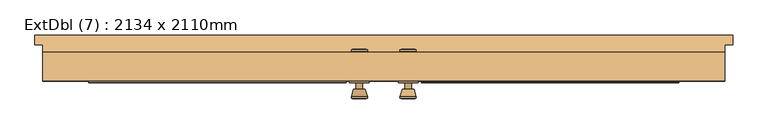
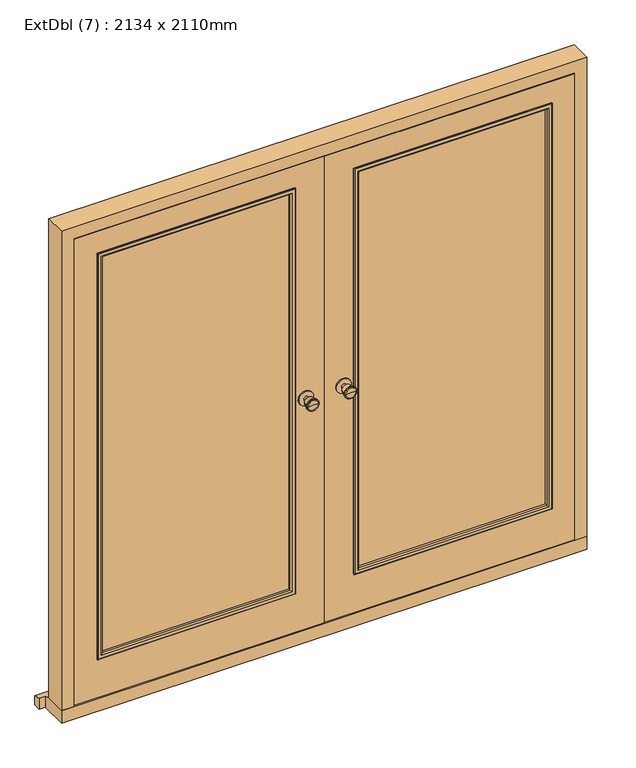
"""IFC4 building model written with IfcOpenShell, lengths in millimetres: door geometry, ExtDbl (7) : 2134 x 2110mm."""

from ifc_helpers import new_model, si_unit, point, frame, frame_2d, origin, place, context, project, spatial, polyline, circle_curve, ellipse_curve, trimmed, segment, composite_curve, outline, extrude, faceted_brep, source, transform, mapped, element, save
from ifc_brep_helpers import plane_surface, cylinder_surface, revolved_surface, advanced_brep


def extdbl_7_2134_x_2110mm_9b31339b(model_context):
    return source(origin(), model_context, "Body", "SolidModel", [
        advanced_brep(
        [(-76.5, -5.7, 1050.0), (-66.5, -5.7, 1050.0), (-86.5, -5.7, 1050.0), (-96.9758676, -54.7, 1050.0), (-56.0241324, -54.7, 1050.0), (-76.5, -54.7, 1050.0), (-101.5, -52.8721319, 1050.0), (-51.5, -52.8721319, 1050.0), (-101.5, -49.4084537, 1050.0), (-51.5, -49.4084537, 1050.0), (-95.136236, -24.7, 1050.0), (-57.863764, -24.7, 1050.0), (-86.5, -24.7, 1050.0), (-66.5, -24.7, 1050.0)],
        [
            (0, 1),
            (1, 2, circle_curve(frame((-76.5, -5.7, 1050.0), z_axis=(0.0, 1.0, 0.0), x_axis=(1.0, 0.0, 0.0)), 10.0)),
            (2, 0),
            (2, 1, circle_curve(frame((-76.5, -5.7, 1050.0), z_axis=(0.0, 1.0, 0.0), x_axis=(1.0, 0.0, 0.0)), 10.0)),
            (3, 4, circle_curve(frame((-76.5, -54.7, 1050.0), z_axis=(0.0, -1.0, 0.0), x_axis=(1.0, 0.0, 0.0)), 20.4758676)),
            (4, 5),
            (5, 3),
            (4, 3, circle_curve(frame((-76.5, -54.7, 1050.0), z_axis=(0.0, -1.0, 0.0), x_axis=(1.0, 0.0, 0.0)), 20.4758676)),
            (6, 7, circle_curve(frame((-76.5, -52.8721319, 1050.0), z_axis=(0.0, -1.0, 0.0), x_axis=(1.0, 0.0, 0.0)), 25.0)),
            (7, 4),
            (3, 6),
            (7, 6, circle_curve(frame((-76.5, -52.8721319, 1050.0), z_axis=(0.0, -1.0, 0.0), x_axis=(1.0, 0.0, 0.0)), 25.0)),
            (8, 9, circle_curve(frame((-76.5, -49.4084537, 1050.0), z_axis=(0.0, -1.0, 0.0), x_axis=(1.0, 0.0, 0.0)), 25.0)),
            (9, 7),
            (6, 8),
            (9, 8, circle_curve(frame((-76.5, -49.4084537, 1050.0), z_axis=(0.0, -1.0, 0.0), x_axis=(1.0, 0.0, 0.0)), 25.0)),
            (10, 11, circle_curve(frame((-76.5, -24.7, 1050.0), z_axis=(0.0, -1.0, 0.0), x_axis=(1.0, 0.0, 0.0)), 18.636236)),
            (11, 9),
            (8, 10),
            (11, 10, circle_curve(frame((-76.5, -24.7, 1050.0), z_axis=(0.0, -1.0, 0.0), x_axis=(1.0, 0.0, 0.0)), 18.636236)),
            (12, 13, circle_curve(frame((-76.5, -24.7, 1050.0), z_axis=(0.0, -1.0, 0.0), x_axis=(1.0, 0.0, 0.0)), 10.0)),
            (13, 11),
            (10, 12),
            (13, 12, circle_curve(frame((-76.5, -24.7, 1050.0), z_axis=(0.0, -1.0, 0.0), x_axis=(1.0, 0.0, 0.0)), 10.0)),
            (1, 13),
            (12, 2),
        ],
        [
            plane_surface(frame((-76.5, -5.7, 1050.0), z_axis=(0.0, 1.0, 0.0), x_axis=(1.0, 0.0, 0.0))),
            plane_surface(frame((-76.5, -54.7, 1050.0), z_axis=(0.0, -1.0, 0.0), x_axis=(1.0, 0.0, 0.0))),
            revolved_surface(polyline([(-56.0241324, -54.7, 1050.0), (-51.5, -52.8721319, 1050.0)]), (-76.5, -5.7, 1050.0), (0.0, 1.0, 0.0)),
            cylinder_surface(frame((-76.5, -5.7, 1050.0), z_axis=(0.0, 1.0, 0.0), x_axis=(1.0, 0.0, 0.0)), 25.0),
            revolved_surface(polyline([(-51.5, -49.4084537, 1050.0), (-57.863764, -24.7, 1050.0)]), (-76.5, -5.7, 1050.0), (0.0, 1.0, 0.0)),
            plane_surface(frame((-76.5, -24.7, 1050.0), z_axis=(0.0, 1.0, 0.0), x_axis=(1.0, 0.0, 0.0))),
            cylinder_surface(frame((-76.5, -5.7, 1050.0), z_axis=(0.0, 1.0, 0.0), x_axis=(1.0, 0.0, 0.0)), 10.0),
        ],
        [
            (0, [[1, 2, 3]]),
            (0, [[-3, 4, -1]]),
            (1, [[5, 6, 7]]),
            (1, [[8, -7, -6]]),
            (2, [[9, 10, -5, 11]]),
            (2, [[12, -11, -8, -10]]),
            (3, [[13, 14, -9, 15]]),
            (3, [[16, -15, -12, -14]]),
            (4, [[17, 18, -13, 19]]),
            (4, [[20, -19, -16, -18]]),
            (5, [[21, 22, -17, 23]]),
            (5, [[24, -23, -20, -22]]),
            (6, [[-2, 25, -21, 26]]),
            (6, [[-4, -26, -24, -25]]),
        ],
    ),
        extrude(outline(composite_curve([segment(trimmed(circle_curve(frame_2d((1050.0, -76.5)), 30.0), [point((1050.0, -46.5))], [point((1050.0, -106.5))], False, "CARTESIAN"), True, "CONTINUOUS"), segment(trimmed(circle_curve(frame_2d((1050.0, -76.5)), 30.0), [point((1050.0, -106.5))], [point((1050.0, -46.5))], False, "CARTESIAN"), True, "CONTINUOUS")], self_intersect=False)), frame((0.0, -5.7, 0.0), z_axis=(0.0, 1.0, 0.0), x_axis=(0.0, 0.0, 1.0)), (0.0, 0.0, 1.0), 6.0),
        advanced_brep(
        [(-76.5, 50.3, 1050.0), (-86.5, 50.3, 1050.0), (-66.5, 50.3, 1050.0), (-96.9758676, 99.3, 1050.0), (-76.5, 99.3, 1050.0), (-56.0241324, 99.3, 1050.0), (-101.5, 97.4721319, 1050.0), (-51.5, 97.4721319, 1050.0), (-101.5, 94.0084537, 1050.0), (-51.5, 94.0084537, 1050.0), (-95.136236, 69.3, 1050.0), (-57.863764, 69.3, 1050.0), (-86.5, 69.3, 1050.0), (-66.5, 69.3, 1050.0)],
        [
            (0, 1),
            (1, 2, circle_curve(frame((-76.5, 50.3, 1050.0), z_axis=(0.0, -1.0, 0.0), x_axis=(1.0, 0.0, 0.0)), 10.0)),
            (2, 0),
            (2, 1, circle_curve(frame((-76.5, 50.3, 1050.0), z_axis=(0.0, -1.0, 0.0), x_axis=(1.0, 0.0, 0.0)), 10.0)),
            (3, 4),
            (4, 5),
            (5, 3, circle_curve(frame((-76.5, 99.3, 1050.0), z_axis=(0.0, 1.0, 0.0), x_axis=(1.0, 0.0, 0.0)), 20.4758676)),
            (3, 5, circle_curve(frame((-76.5, 99.3, 1050.0), z_axis=(0.0, 1.0, 0.0), x_axis=(1.0, 0.0, 0.0)), 20.4758676)),
            (6, 3),
            (5, 7),
            (7, 6, circle_curve(frame((-76.5, 97.4721319, 1050.0), z_axis=(0.0, 1.0, 0.0), x_axis=(1.0, 0.0, 0.0)), 25.0)),
            (6, 7, circle_curve(frame((-76.5, 97.4721319, 1050.0), z_axis=(0.0, 1.0, 0.0), x_axis=(1.0, 0.0, 0.0)), 25.0)),
            (8, 6),
            (7, 9),
            (9, 8, circle_curve(frame((-76.5, 94.0084537, 1050.0), z_axis=(0.0, 1.0, 0.0), x_axis=(1.0, 0.0, 0.0)), 25.0)),
            (8, 9, circle_curve(frame((-76.5, 94.0084537, 1050.0), z_axis=(0.0, 1.0, 0.0), x_axis=(1.0, 0.0, 0.0)), 25.0)),
            (10, 8),
            (9, 11),
            (11, 10, circle_curve(frame((-76.5, 69.3, 1050.0), z_axis=(0.0, 1.0, 0.0), x_axis=(1.0, 0.0, 0.0)), 18.636236)),
            (10, 11, circle_curve(frame((-76.5, 69.3, 1050.0), z_axis=(0.0, 1.0, 0.0), x_axis=(1.0, 0.0, 0.0)), 18.636236)),
            (12, 10),
            (11, 13),
            (13, 12, circle_curve(frame((-76.5, 69.3, 1050.0), z_axis=(0.0, 1.0, 0.0), x_axis=(1.0, 0.0, 0.0)), 10.0)),
            (12, 13, circle_curve(frame((-76.5, 69.3, 1050.0), z_axis=(0.0, 1.0, 0.0), x_axis=(1.0, 0.0, 0.0)), 10.0)),
            (1, 12),
            (13, 2),
        ],
        [
            plane_surface(frame((-76.5, 50.3, 1050.0), z_axis=(0.0, -1.0, 0.0), x_axis=(1.0, 0.0, 0.0))),
            plane_surface(frame((-76.5, 99.3, 1050.0), z_axis=(0.0, 1.0, 0.0), x_axis=(1.0, 0.0, 0.0))),
            revolved_surface(polyline([(-56.0241324, 99.3, 1050.0), (-51.5, 97.4721319, 1050.0)]), (-76.5, 50.3, 1050.0), (0.0, -1.0, 0.0)),
            cylinder_surface(frame((-76.5, 50.3, 1050.0), z_axis=(0.0, -1.0, 0.0), x_axis=(1.0, 0.0, 0.0)), 25.0),
            revolved_surface(polyline([(-51.5, 94.0084537, 1050.0), (-57.863764, 69.3, 1050.0)]), (-76.5, 50.3, 1050.0), (0.0, -1.0, 0.0)),
            plane_surface(frame((-76.5, 69.3, 1050.0), z_axis=(0.0, -1.0, 0.0), x_axis=(1.0, 0.0, 0.0))),
            cylinder_surface(frame((-76.5, 50.3, 1050.0), z_axis=(0.0, -1.0, 0.0), x_axis=(1.0, 0.0, 0.0)), 10.0),
        ],
        [
            (0, [[1, 2, 3]]),
            (0, [[-3, 4, -1]]),
            (1, [[5, 6, 7]]),
            (1, [[-6, -5, 8]]),
            (2, [[9, -7, 10, 11]]),
            (2, [[-10, -8, -9, 12]]),
            (3, [[13, -11, 14, 15]]),
            (3, [[-14, -12, -13, 16]]),
            (4, [[17, -15, 18, 19]]),
            (4, [[-18, -16, -17, 20]]),
            (5, [[21, -19, 22, 23]]),
            (5, [[-22, -20, -21, 24]]),
            (6, [[25, -23, 26, -2]]),
            (6, [[-26, -24, -25, -4]]),
        ],
    ),
        extrude(outline(composite_curve([segment(trimmed(circle_curve(frame_2d((1050.0, -76.5)), 30.0), [point((1050.0, -46.5))], [point((1050.0, -106.5))], False, "CARTESIAN"), True, "CONTINUOUS"), segment(trimmed(circle_curve(frame_2d((1050.0, -76.5)), 30.0), [point((1050.0, -106.5))], [point((1050.0, -46.5))], False, "CARTESIAN"), True, "CONTINUOUS")], self_intersect=False)), frame((0.0, 44.3, 0.0), z_axis=(0.0, 1.0, 0.0), x_axis=(0.0, 0.0, 1.0)), (0.0, 0.0, 1.0), 6.0),
        advanced_brep(
        [(76.5, -5.7, 1050.0), (86.5, -5.7, 1050.0), (66.5, -5.7, 1050.0), (96.9758676, -54.7, 1050.0), (76.5, -54.7, 1050.0), (56.0241324, -54.7, 1050.0), (101.5, -52.8721319, 1050.0), (51.5, -52.8721319, 1050.0), (101.5, -49.4084537, 1050.0), (51.5, -49.4084537, 1050.0), (95.136236, -24.7, 1050.0), (57.863764, -24.7, 1050.0), (86.5, -24.7, 1050.0), (66.5, -24.7, 1050.0)],
        [
            (0, 1),
            (1, 2, circle_curve(frame((76.5, -5.7, 1050.0), z_axis=(0.0, 1.0, 0.0), x_axis=(-1.0, 0.0, 0.0)), 10.0)),
            (2, 0),
            (2, 1, circle_curve(frame((76.5, -5.7, 1050.0), z_axis=(0.0, 1.0, 0.0), x_axis=(-1.0, 0.0, 0.0)), 10.0)),
            (3, 4),
            (4, 5),
            (5, 3, circle_curve(frame((76.5, -54.7, 1050.0), z_axis=(0.0, -1.0, 0.0), x_axis=(-1.0, 0.0, 0.0)), 20.4758676)),
            (3, 5, circle_curve(frame((76.5, -54.7, 1050.0), z_axis=(0.0, -1.0, 0.0), x_axis=(-1.0, 0.0, 0.0)), 20.4758676)),
            (6, 3),
            (5, 7),
            (7, 6, circle_curve(frame((76.5, -52.8721319, 1050.0), z_axis=(0.0, -1.0, 0.0), x_axis=(-1.0, 0.0, 0.0)), 25.0)),
            (6, 7, circle_curve(frame((76.5, -52.8721319, 1050.0), z_axis=(0.0, -1.0, 0.0), x_axis=(-1.0, 0.0, 0.0)), 25.0)),
            (8, 6),
            (7, 9),
            (9, 8, circle_curve(frame((76.5, -49.4084537, 1050.0), z_axis=(0.0, -1.0, 0.0), x_axis=(-1.0, 0.0, 0.0)), 25.0)),
            (8, 9, circle_curve(frame((76.5, -49.4084537, 1050.0), z_axis=(0.0, -1.0, 0.0), x_axis=(-1.0, 0.0, 0.0)), 25.0)),
            (10, 8),
            (9, 11),
            (11, 10, circle_curve(frame((76.5, -24.7, 1050.0), z_axis=(0.0, -1.0, 0.0), x_axis=(-1.0, 0.0, 0.0)), 18.636236)),
            (10, 11, circle_curve(frame((76.5, -24.7, 1050.0), z_axis=(0.0, -1.0, 0.0), x_axis=(-1.0, 0.0, 0.0)), 18.636236)),
            (12, 10),
            (11, 13),
            (13, 12, circle_curve(frame((76.5, -24.7, 1050.0), z_axis=(0.0, -1.0, 0.0), x_axis=(-1.0, 0.0, 0.0)), 10.0)),
            (12, 13, circle_curve(frame((76.5, -24.7, 1050.0), z_axis=(0.0, -1.0, 0.0), x_axis=(-1.0, 0.0, 0.0)), 10.0)),
            (1, 12),
            (13, 2),
        ],
        [
            plane_surface(frame((76.5, -5.7, 1050.0), z_axis=(0.0, 1.0, 0.0), x_axis=(-1.0, 0.0, 0.0))),
            plane_surface(frame((76.5, -54.7, 1050.0), z_axis=(0.0, -1.0, 0.0), x_axis=(-1.0, 0.0, 0.0))),
            revolved_surface(polyline([(56.0241324, -54.7, 1050.0), (51.5, -52.8721319, 1050.0)]), (76.5, -5.7, 1050.0), (0.0, 1.0, 0.0)),
            cylinder_surface(frame((76.5, -5.7, 1050.0), z_axis=(0.0, 1.0, 0.0), x_axis=(-1.0, 0.0, 0.0)), 25.0),
            revolved_surface(polyline([(51.5, -49.4084537, 1050.0), (57.863764, -24.7, 1050.0)]), (76.5, -5.7, 1050.0), (0.0, 1.0, 0.0)),
            plane_surface(frame((76.5, -24.7, 1050.0), z_axis=(0.0, 1.0, 0.0), x_axis=(-1.0, 0.0, 0.0))),
            cylinder_surface(frame((76.5, -5.7, 1050.0), z_axis=(0.0, 1.0, 0.0), x_axis=(-1.0, 0.0, 0.0)), 10.0),
        ],
        [
            (0, [[1, 2, 3]]),
            (0, [[-3, 4, -1]]),
            (1, [[5, 6, 7]]),
            (1, [[-6, -5, 8]]),
            (2, [[9, -7, 10, 11]]),
            (2, [[-10, -8, -9, 12]]),
            (3, [[13, -11, 14, 15]]),
            (3, [[-14, -12, -13, 16]]),
            (4, [[17, -15, 18, 19]]),
            (4, [[-18, -16, -17, 20]]),
            (5, [[21, -19, 22, 23]]),
            (5, [[-22, -20, -21, 24]]),
            (6, [[25, -23, 26, -2]]),
            (6, [[-26, -24, -25, -4]]),
        ],
    ),
        extrude(outline(composite_curve([segment(trimmed(circle_curve(frame_2d((1050.0, 76.5)), 30.0), [point((1050.0, 46.5))], [point((1050.0, 106.5))], False, "CARTESIAN"), True, "CONTINUOUS"), segment(trimmed(circle_curve(frame_2d((1050.0, 76.5)), 30.0), [point((1050.0, 106.5))], [point((1050.0, 46.5))], False, "CARTESIAN"), True, "CONTINUOUS")], self_intersect=False)), frame((0.0, -5.7, 0.0), z_axis=(0.0, 1.0, 0.0), x_axis=(0.0, 0.0, 1.0)), (0.0, 0.0, 1.0), 6.0),
        advanced_brep(
        [(76.5, 50.3, 1050.0), (66.5, 50.3, 1050.0), (86.5, 50.3, 1050.0), (96.9758676, 99.3, 1050.0), (56.0241324, 99.3, 1050.0), (76.5, 99.3, 1050.0), (101.5, 97.4721319, 1050.0), (51.5, 97.4721319, 1050.0), (101.5, 94.0084537, 1050.0), (51.5, 94.0084537, 1050.0), (95.136236, 69.3, 1050.0), (57.863764, 69.3, 1050.0), (86.5, 69.3, 1050.0), (66.5, 69.3, 1050.0)],
        [
            (0, 1),
            (1, 2, circle_curve(frame((76.5, 50.3, 1050.0), z_axis=(0.0, -1.0, 0.0), x_axis=(-1.0, 0.0, 0.0)), 10.0)),
            (2, 0),
            (2, 1, circle_curve(frame((76.5, 50.3, 1050.0), z_axis=(0.0, -1.0, 0.0), x_axis=(-1.0, 0.0, 0.0)), 10.0)),
            (3, 4, circle_curve(frame((76.5, 99.3, 1050.0), z_axis=(0.0, 1.0, 0.0), x_axis=(-1.0, 0.0, 0.0)), 20.4758676)),
            (4, 5),
            (5, 3),
            (4, 3, circle_curve(frame((76.5, 99.3, 1050.0), z_axis=(0.0, 1.0, 0.0), x_axis=(-1.0, 0.0, 0.0)), 20.4758676)),
            (6, 7, circle_curve(frame((76.5, 97.4721319, 1050.0), z_axis=(0.0, 1.0, 0.0), x_axis=(-1.0, 0.0, 0.0)), 25.0)),
            (7, 4),
            (3, 6),
            (7, 6, circle_curve(frame((76.5, 97.4721319, 1050.0), z_axis=(0.0, 1.0, 0.0), x_axis=(-1.0, 0.0, 0.0)), 25.0)),
            (8, 9, circle_curve(frame((76.5, 94.0084537, 1050.0), z_axis=(0.0, 1.0, 0.0), x_axis=(-1.0, 0.0, 0.0)), 25.0)),
            (9, 7),
            (6, 8),
            (9, 8, circle_curve(frame((76.5, 94.0084537, 1050.0), z_axis=(0.0, 1.0, 0.0), x_axis=(-1.0, 0.0, 0.0)), 25.0)),
            (10, 11, circle_curve(frame((76.5, 69.3, 1050.0), z_axis=(0.0, 1.0, 0.0), x_axis=(-1.0, 0.0, 0.0)), 18.636236)),
            (11, 9),
            (8, 10),
            (11, 10, circle_curve(frame((76.5, 69.3, 1050.0), z_axis=(0.0, 1.0, 0.0), x_axis=(-1.0, 0.0, 0.0)), 18.636236)),
            (12, 13, circle_curve(frame((76.5, 69.3, 1050.0), z_axis=(0.0, 1.0, 0.0), x_axis=(-1.0, 0.0, 0.0)), 10.0)),
            (13, 11),
            (10, 12),
            (13, 12, circle_curve(frame((76.5, 69.3, 1050.0), z_axis=(0.0, 1.0, 0.0), x_axis=(-1.0, 0.0, 0.0)), 10.0)),
            (1, 13),
            (12, 2),
        ],
        [
            plane_surface(frame((76.5, 50.3, 1050.0), z_axis=(0.0, -1.0, 0.0), x_axis=(-1.0, 0.0, 0.0))),
            plane_surface(frame((76.5, 99.3, 1050.0), z_axis=(0.0, 1.0, 0.0), x_axis=(-1.0, 0.0, 0.0))),
            revolved_surface(polyline([(56.0241324, 99.3, 1050.0), (51.5, 97.4721319, 1050.0)]), (76.5, 50.3, 1050.0), (0.0, -1.0, 0.0)),
            cylinder_surface(frame((76.5, 50.3, 1050.0), z_axis=(0.0, -1.0, 0.0), x_axis=(-1.0, 0.0, 0.0)), 25.0),
            revolved_surface(polyline([(51.5, 94.0084537, 1050.0), (57.863764, 69.3, 1050.0)]), (76.5, 50.3, 1050.0), (0.0, -1.0, 0.0)),
            plane_surface(frame((76.5, 69.3, 1050.0), z_axis=(0.0, -1.0, 0.0), x_axis=(-1.0, 0.0, 0.0))),
            cylinder_surface(frame((76.5, 50.3, 1050.0), z_axis=(0.0, -1.0, 0.0), x_axis=(-1.0, 0.0, 0.0)), 10.0),
        ],
        [
            (0, [[1, 2, 3]]),
            (0, [[-3, 4, -1]]),
            (1, [[5, 6, 7]]),
            (1, [[8, -7, -6]]),
            (2, [[9, 10, -5, 11]]),
            (2, [[12, -11, -8, -10]]),
            (3, [[13, 14, -9, 15]]),
            (3, [[16, -15, -12, -14]]),
            (4, [[17, 18, -13, 19]]),
            (4, [[20, -19, -16, -18]]),
            (5, [[21, 22, -17, 23]]),
            (5, [[24, -23, -20, -22]]),
            (6, [[-2, 25, -21, 26]]),
            (6, [[-4, -26, -24, -25]]),
        ],
    ),
        extrude(outline(composite_curve([segment(trimmed(circle_curve(frame_2d((1050.0, 76.5)), 30.0), [point((1050.0, 46.5))], [point((1050.0, 106.5))], False, "CARTESIAN"), True, "CONTINUOUS"), segment(trimmed(circle_curve(frame_2d((1050.0, 76.5)), 30.0), [point((1050.0, 106.5))], [point((1050.0, 46.5))], False, "CARTESIAN"), True, "CONTINUOUS")], self_intersect=False)), frame((0.0, 44.3, 0.0), z_axis=(0.0, 1.0, 0.0), x_axis=(0.0, 0.0, 1.0)), (0.0, 0.0, 1.0), 6.0),
        faceted_brep([(996.3, 89.3, 54.5), (1066.8, 89.3, 54.5), (1066.8, 0.3, 54.5), (1018.3, 0.3, 54.5), (1018.3, 47.3, 54.5), (996.3, 47.3, 54.5), (996.3, 89.3, 2039.5), (-996.3, 89.3, 2039.5), (-996.3, 89.3, 54.5), (-1066.8, 89.3, 54.5), (-1066.8, 89.3, 2110.0), (1066.8, 89.3, 2110.0), (1066.8, 0.3, 2110.0), (-1066.8, 0.3, 2110.0), (-1066.8, 0.3, 54.5), (-1018.3, 0.3, 54.5), (-1018.3, 0.3, 2061.5), (1018.3, 0.3, 2061.5), (1018.3, 47.3, 2061.5), (-1018.3, 47.3, 2061.5), (-1018.3, 47.3, 54.5), (-996.3, 47.3, 54.5), (-996.3, 47.3, 2039.5), (996.3, 47.3, 2039.5)], [[[0, 1, 2, 3, 4, 5]], [[1, 0, 6, 7, 8, 9, 10, 11]], [[2, 1, 11, 12]], [[3, 2, 12, 13, 14, 15, 16, 17]], [[4, 3, 17, 18]], [[5, 4, 18, 19, 20, 21, 22, 23]], [[0, 5, 23, 6]], [[7, 22, 21, 8]], [[8, 21, 20, 15, 14, 9]], [[13, 10, 9, 14]], [[19, 16, 15, 20]], [[12, 11, 10, 13]], [[18, 17, 16, 19]], [[6, 23, 22, 7]]]),
        extrude(outline(polyline([(58.5, 1015.3), (2058.5, 1015.3), (2058.5, 1.5), (58.5, 1.5), (58.5, 1015.3)]), holes=[polyline([(1958.5, 915.3), (233.5, 915.3), (233.5, 126.5), (1958.5, 126.5), (1958.5, 915.3)])]), frame((0.0, 0.3, 0.0), z_axis=(0.0, 1.0, 0.0), x_axis=(0.0, 0.0, 1.0)), (0.0, 0.0, 1.0), 44.0),
        extrude(outline(polyline([(58.5, -1015.3), (58.5, -1.5), (2058.5, -1.5), (2058.5, -1015.3), (58.5, -1015.3)]), holes=[polyline([(1958.5, -126.5), (233.5, -126.5), (233.5, -915.3), (1958.5, -915.3), (1958.5, -126.5)])]), frame((0.0, 0.3, 0.0), z_axis=(0.0, 1.0, 0.0), x_axis=(0.0, 0.0, 1.0)), (0.0, 0.0, 1.0), 44.0),
        faceted_brep([(1091.8, 144.3, 0.0), (1091.8, 144.3, 38.5947221), (1091.8, 114.3, 47.2703282), (1091.8, 114.3, 0.0), (-1091.8, 144.3, 38.5947221), (-1091.8, 144.3, 0.0), (-1091.8, 114.3, 0.0), (-1091.8, 114.3, 47.2703282), (1066.8, 114.3, 0.0), (1066.8, 0.3, 0.0), (-1066.8, 0.3, 0.0), (-1066.8, 114.3, 0.0), (-1066.8, 114.3, 47.2703282), (-1066.8, 89.3, 54.5), (1066.8, 89.3, 54.5), (1066.8, 114.3, 47.2703282), (-1066.8, 0.3, 54.5), (1066.8, 0.3, 54.5)], [[[0, 1, 2, 3]], [[4, 5, 6, 7]], [[5, 0, 3, 8, 9, 10, 11, 6]], [[1, 0, 5, 4]], [[1, 4, 7, 12, 13, 14, 15, 2]], [[13, 16, 17, 14]], [[16, 10, 9, 17]], [[12, 11, 10, 16, 13]], [[11, 12, 7, 6]], [[8, 15, 14, 17, 9]], [[15, 8, 3, 2]]]),
        extrude(outline(polyline([(126.5, 34.3), (915.3, 34.3), (915.3, 10.3), (126.5, 10.3), (126.5, 34.3)])), frame((0.0, 0.0, 233.5), z_axis=(0.0, 0.0, 1.0), x_axis=(1.0, 0.0, 0.0)), (0.0, 0.0, 1.0), 1725.0),
        extrude(outline(polyline([(-915.3, 34.3), (-126.5, 34.3), (-126.5, 10.3), (-915.3, 10.3), (-915.3, 34.3)])), frame((0.0, 0.0, 233.5), z_axis=(0.0, 0.0, 1.0), x_axis=(1.0, 0.0, 0.0)), (0.0, 0.0, 1.0), 1725.0),
        advanced_brep(
        [(118.5, 48.3, 225.5), (118.5, 44.3, 225.5), (118.5, 44.3, 1966.5), (118.5, 48.3, 1966.5), (120.5, 50.3, 227.5), (120.5, 50.3, 1964.5), (138.5, 45.3, 245.5), (133.5, 50.3, 240.5), (133.5, 50.3, 1951.5), (138.5, 45.3, 1946.5), (138.5, 34.3, 245.5), (138.5, 34.3, 1946.5), (126.5, 44.3, 233.5), (126.5, 34.3, 233.5), (126.5, 34.3, 1958.5), (126.5, 44.3, 1958.5), (923.3, 44.3, 1966.5), (923.3, 48.3, 1966.5), (921.3, 50.3, 1964.5), (908.3, 50.3, 1951.5), (903.3, 45.3, 1946.5), (903.3, 34.3, 1946.5), (915.3, 34.3, 1958.5), (915.3, 44.3, 1958.5), (923.3, 44.3, 225.5), (923.3, 48.3, 225.5), (921.3, 50.3, 227.5), (908.3, 50.3, 240.5), (903.3, 45.3, 245.5), (903.3, 34.3, 245.5), (915.3, 34.3, 233.5), (915.3, 44.3, 233.5)],
        [
            (0, 1),
            (1, 2),
            (2, 3),
            (3, 0),
            (4, 0, ellipse_curve(frame((120.5, 48.3, 227.5), z_axis=(-0.7071067811865476, 0.0, 0.7071067811865475), x_axis=(-0.7071067811865475, 0.0, -0.7071067811865476)), 2.8284271, 2.0)),
            (3, 5, ellipse_curve(frame((120.5, 48.3, 1964.5), z_axis=(-0.7071067811865475, 0.0, -0.7071067811865476), x_axis=(0.7071067811865475, 0.0, -0.7071067811865475)), 2.8284271, 2.0)),
            (5, 4),
            (6, 7, ellipse_curve(frame((133.5, 45.3, 240.5), z_axis=(-0.7071067811865476, 0.0, 0.7071067811865475), x_axis=(-0.7071067811865475, 0.0, -0.7071067811865476)), 7.0710678, 5.0)),
            (7, 8),
            (8, 9, ellipse_curve(frame((133.5, 45.3, 1951.5), z_axis=(-0.7071067811865475, 0.0, -0.7071067811865476), x_axis=(0.7071067811865475, 0.0, -0.7071067811865475)), 7.0710678, 5.0)),
            (9, 6),
            (10, 6),
            (9, 11),
            (11, 10),
            (12, 13),
            (13, 14),
            (14, 15),
            (15, 12),
            (2, 16),
            (16, 17),
            (17, 3),
            (17, 18, ellipse_curve(frame((921.3, 48.3, 1964.5), z_axis=(-0.7071067811865475, 0.0, 0.7071067811865475), x_axis=(-0.7071067811865477, 0.0, -0.7071067811865472)), 2.8284271, 2.0)),
            (18, 5),
            (8, 19),
            (19, 20, ellipse_curve(frame((908.3, 45.3, 1951.5), z_axis=(-0.7071067811865475, 0.0, 0.7071067811865475), x_axis=(-0.7071067811865477, 0.0, -0.7071067811865472)), 7.0710678, 5.0)),
            (20, 9),
            (20, 21),
            (21, 11),
            (14, 22),
            (22, 23),
            (23, 15),
            (16, 24),
            (24, 25),
            (25, 17),
            (25, 26, ellipse_curve(frame((921.3, 48.3, 227.5), z_axis=(0.7071067811865475, 0.0, 0.7071067811865475), x_axis=(-0.7071067811865475, 0.0, 0.7071067811865476)), 2.8284271, 2.0)),
            (26, 18),
            (19, 27),
            (27, 28, ellipse_curve(frame((908.3, 45.3, 240.5), z_axis=(0.7071067811865475, 0.0, 0.7071067811865475), x_axis=(-0.7071067811865475, 0.0, 0.7071067811865476)), 7.0710678, 5.0)),
            (28, 20),
            (28, 29),
            (29, 21),
            (22, 30),
            (30, 31),
            (31, 23),
            (24, 1),
            (0, 25),
            (4, 26),
            (7, 27),
            (6, 28),
            (10, 29),
            (13, 30),
            (12, 31),
        ],
        [
            plane_surface(frame((118.5, 44.3, 225.5), z_axis=(-1.0, 0.0, 0.0), x_axis=(0.0, 0.0, 1.0))),
            cylinder_surface(frame((120.5, 48.3, 233.5), z_axis=(0.0, 0.0, -1.0), x_axis=(-1.0, 0.0, 0.0)), 2.0),
            cylinder_surface(frame((133.5, 45.3, 233.5), z_axis=(0.0, 0.0, -1.0), x_axis=(-1.0, 0.0, 0.0)), 5.0),
            plane_surface(frame((138.5, 45.3, 245.5), z_axis=(1.0, 0.0, 0.0), x_axis=(0.0, 0.0, 1.0))),
            plane_surface(frame((126.5, 34.3, 233.5), z_axis=(-1.0, 0.0, 0.0), x_axis=(0.0, 0.0, 1.0))),
            plane_surface(frame((118.5, 44.3, 1966.5), z_axis=(0.0, 0.0, 1.0), x_axis=(1.0, 0.0, 0.0))),
            cylinder_surface(frame((126.5, 48.3, 1964.5), z_axis=(-1.0, 0.0, 0.0), x_axis=(0.0, 0.0, 1.0)), 2.0),
            cylinder_surface(frame((126.5, 45.3, 1951.5), z_axis=(-1.0, 0.0, 0.0), x_axis=(0.0, 0.0, 1.0)), 5.0),
            plane_surface(frame((138.5, 45.3, 1946.5), z_axis=(0.0, 0.0, -1.0), x_axis=(1.0, 0.0, 0.0))),
            plane_surface(frame((126.5, 34.3, 1958.5), z_axis=(0.0, 0.0, 1.0), x_axis=(1.0, 0.0, 0.0))),
            plane_surface(frame((923.3, 44.3, 1966.5), z_axis=(1.0, 0.0, 0.0), x_axis=(0.0, 0.0, -1.0))),
            cylinder_surface(frame((921.3, 48.3, 1958.5), z_axis=(0.0, 0.0, 1.0), x_axis=(1.0, 0.0, 0.0)), 2.0),
            cylinder_surface(frame((908.3, 45.3, 1958.5), z_axis=(0.0, 0.0, 1.0), x_axis=(1.0, 0.0, 0.0)), 5.0),
            plane_surface(frame((903.3, 45.3, 1946.5), z_axis=(-1.0, 0.0, 0.0), x_axis=(0.0, 0.0, -1.0))),
            plane_surface(frame((915.3, 34.3, 1958.5), z_axis=(1.0, 0.0, 0.0), x_axis=(0.0, 0.0, -1.0))),
            plane_surface(frame((923.3, 44.3, 225.5), z_axis=(0.0, 0.0, -1.0), x_axis=(-1.0, 0.0, 0.0))),
            cylinder_surface(frame((915.3, 48.3, 227.5), z_axis=(1.0, 0.0, 0.0), x_axis=(0.0, 0.0, -1.0)), 2.0),
            plane_surface(frame((921.3, 50.3, 227.5), z_axis=(0.0, 1.0, 0.0), x_axis=(-1.0, 0.0, 0.0))),
            cylinder_surface(frame((915.3, 45.3, 240.5), z_axis=(1.0, 0.0, 0.0), x_axis=(0.0, 0.0, -1.0)), 5.0),
            plane_surface(frame((903.3, 45.3, 245.5), z_axis=(0.0, 0.0, 1.0), x_axis=(-1.0, 0.0, 0.0))),
            plane_surface(frame((903.3, 34.3, 245.5), z_axis=(0.0, -1.0, 0.0), x_axis=(-1.0, 0.0, 0.0))),
            plane_surface(frame((915.3, 34.3, 233.5), z_axis=(0.0, 0.0, -1.0), x_axis=(-1.0, 0.0, 0.0))),
            plane_surface(frame((915.3, 44.3, 233.5), z_axis=(0.0, -1.0, 0.0), x_axis=(-1.0, 0.0, 0.0))),
        ],
        [
            (0, [[1, 2, 3, 4]]),
            (1, [[5, -4, 6, 7]]),
            (2, [[8, 9, 10, 11]]),
            (3, [[12, -11, 13, 14]]),
            (4, [[15, 16, 17, 18]]),
            (5, [[-3, 19, 20, 21]]),
            (6, [[-6, -21, 22, 23]]),
            (7, [[-10, 24, 25, 26]]),
            (8, [[-13, -26, 27, 28]]),
            (9, [[-17, 29, 30, 31]]),
            (10, [[-20, 32, 33, 34]]),
            (11, [[-22, -34, 35, 36]]),
            (12, [[-25, 37, 38, 39]]),
            (13, [[-27, -39, 40, 41]]),
            (14, [[-30, 42, 43, 44]]),
            (15, [[-33, 45, -1, 46]]),
            (16, [[-35, -46, -5, 47]]),
            (17, [[-23, -36, -47, -7], [48, -37, -24, -9]]),
            (18, [[-38, -48, -8, 49]]),
            (19, [[-40, -49, -12, 50]]),
            (20, [[51, -42, -29, -16], [-28, -41, -50, -14]]),
            (21, [[-43, -51, -15, 52]]),
            (22, [[-45, -32, -19, -2], [-31, -44, -52, -18]]),
        ],
    ),
        advanced_brep(
        [(915.3, 10.3, 1958.5), (915.3, 0.3, 1958.5), (915.3, 0.3, 233.5), (915.3, 10.3, 233.5), (903.3, -0.7, 1946.5), (903.3, 10.3, 1946.5), (903.3, 10.3, 245.5), (903.3, -0.7, 245.5), (908.3, -5.7, 1951.5), (908.3, -5.7, 240.5), (923.3, -3.7, 1966.5), (921.3, -5.7, 1964.5), (921.3, -5.7, 227.5), (923.3, -3.7, 225.5), (923.3, 0.3, 1966.5), (923.3, 0.3, 225.5), (126.5, 0.3, 233.5), (126.5, 10.3, 233.5), (138.5, 10.3, 245.5), (138.5, -0.7, 245.5), (133.5, -5.7, 240.5), (120.5, -5.7, 227.5), (118.5, -3.7, 225.5), (118.5, 0.3, 225.5), (126.5, 0.3, 1958.5), (126.5, 10.3, 1958.5), (138.5, 10.3, 1946.5), (138.5, -0.7, 1946.5), (133.5, -5.7, 1951.5), (120.5, -5.7, 1964.5), (118.5, -3.7, 1966.5), (118.5, 0.3, 1966.5)],
        [
            (0, 1),
            (1, 2),
            (2, 3),
            (3, 0),
            (4, 5),
            (5, 6),
            (6, 7),
            (7, 4),
            (8, 4, ellipse_curve(frame((908.3, -0.7, 1951.5), z_axis=(0.7071067811865475, 0.0, -0.7071067811865475), x_axis=(0.7071067811865474, 0.0, 0.7071067811865476)), 7.0710678, 5.0)),
            (7, 9, ellipse_curve(frame((908.3, -0.7, 240.5), z_axis=(0.7071067811865475, 0.0, 0.7071067811865475), x_axis=(-0.7071067811865474, 0.0, 0.7071067811865476)), 7.0710678, 5.0)),
            (9, 8),
            (10, 11, ellipse_curve(frame((921.3, -3.7, 1964.5), z_axis=(0.7071067811865475, 0.0, -0.7071067811865475), x_axis=(0.7071067811865474, 0.0, 0.7071067811865476)), 2.8284271, 2.0)),
            (11, 12),
            (12, 13, ellipse_curve(frame((921.3, -3.7, 227.5), z_axis=(0.7071067811865475, 0.0, 0.7071067811865475), x_axis=(-0.7071067811865474, 0.0, 0.7071067811865476)), 2.8284271, 2.0)),
            (13, 10),
            (14, 10),
            (13, 15),
            (15, 14),
            (2, 16),
            (16, 17),
            (17, 3),
            (6, 18),
            (18, 19),
            (19, 7),
            (19, 20, ellipse_curve(frame((133.5, -0.7, 240.5), z_axis=(0.7071067811865475, 0.0, -0.7071067811865475), x_axis=(0.7071067811865476, 0.0, 0.7071067811865474)), 7.0710678, 5.0)),
            (20, 9),
            (12, 21),
            (21, 22, ellipse_curve(frame((120.5, -3.7, 227.5), z_axis=(0.7071067811865475, 0.0, -0.7071067811865475), x_axis=(0.7071067811865476, 0.0, 0.7071067811865474)), 2.8284271, 2.0)),
            (22, 13),
            (22, 23),
            (23, 15),
            (16, 24),
            (24, 25),
            (25, 17),
            (18, 26),
            (26, 27),
            (27, 19),
            (27, 28, ellipse_curve(frame((133.5, -0.7, 1951.5), z_axis=(-0.7071067811865475, 0.0, -0.7071067811865475), x_axis=(0.7071067811865474, 0.0, -0.7071067811865476)), 7.0710678, 5.0)),
            (28, 20),
            (21, 29),
            (29, 30, ellipse_curve(frame((120.5, -3.7, 1964.5), z_axis=(-0.7071067811865475, 0.0, -0.7071067811865475), x_axis=(0.7071067811865474, 0.0, -0.7071067811865476)), 2.8284271, 2.0)),
            (30, 22),
            (30, 31),
            (31, 23),
            (31, 14),
            (1, 24),
            (0, 25),
            (5, 26),
            (4, 27),
            (8, 28),
            (11, 29),
            (10, 30),
        ],
        [
            plane_surface(frame((915.3, 0.3, 1958.5), z_axis=(1.0, 0.0, 0.0), x_axis=(0.0, 0.0, -1.0))),
            plane_surface(frame((903.3, 10.3, 1946.5), z_axis=(-1.0, 0.0, 0.0), x_axis=(0.0, 0.0, -1.0))),
            cylinder_surface(frame((908.3, -0.7, 1958.5), z_axis=(0.0, 0.0, 1.0), x_axis=(1.0, 0.0, 0.0)), 5.0),
            cylinder_surface(frame((921.3, -3.7, 1958.5), z_axis=(0.0, 0.0, 1.0), x_axis=(1.0, 0.0, 0.0)), 2.0),
            plane_surface(frame((923.3, -3.7, 1966.5), z_axis=(1.0, 0.0, 0.0), x_axis=(0.0, 0.0, -1.0))),
            plane_surface(frame((915.3, 0.3, 233.5), z_axis=(0.0, 0.0, -1.0), x_axis=(-1.0, 0.0, 0.0))),
            plane_surface(frame((903.3, 10.3, 245.5), z_axis=(0.0, 0.0, 1.0), x_axis=(-1.0, 0.0, 0.0))),
            cylinder_surface(frame((915.3, -0.7, 240.5), z_axis=(1.0, 0.0, 0.0), x_axis=(0.0, 0.0, -1.0)), 5.0),
            cylinder_surface(frame((915.3, -3.7, 227.5), z_axis=(1.0, 0.0, 0.0), x_axis=(0.0, 0.0, -1.0)), 2.0),
            plane_surface(frame((923.3, -3.7, 225.5), z_axis=(0.0, 0.0, -1.0), x_axis=(-1.0, 0.0, 0.0))),
            plane_surface(frame((126.5, 0.3, 233.5), z_axis=(-1.0, 0.0, 0.0), x_axis=(0.0, 0.0, 1.0))),
            plane_surface(frame((138.5, 10.3, 245.5), z_axis=(1.0, 0.0, 0.0), x_axis=(0.0, 0.0, 1.0))),
            cylinder_surface(frame((133.5, -0.7, 233.5), z_axis=(0.0, 0.0, -1.0), x_axis=(-1.0, 0.0, 0.0)), 5.0),
            cylinder_surface(frame((120.5, -3.7, 233.5), z_axis=(0.0, 0.0, -1.0), x_axis=(-1.0, 0.0, 0.0)), 2.0),
            plane_surface(frame((118.5, -3.7, 225.5), z_axis=(-1.0, 0.0, 0.0), x_axis=(0.0, 0.0, 1.0))),
            plane_surface(frame((118.5, 0.3, 1966.5), z_axis=(0.0, 1.0, 0.0), x_axis=(1.0, 0.0, 0.0))),
            plane_surface(frame((126.5, 0.3, 1958.5), z_axis=(0.0, 0.0, 1.0), x_axis=(1.0, 0.0, 0.0))),
            plane_surface(frame((126.5, 10.3, 1958.5), z_axis=(0.0, 1.0, 0.0), x_axis=(1.0, 0.0, 0.0))),
            plane_surface(frame((138.5, 10.3, 1946.5), z_axis=(0.0, 0.0, -1.0), x_axis=(1.0, 0.0, 0.0))),
            cylinder_surface(frame((126.5, -0.7, 1951.5), z_axis=(-1.0, 0.0, 0.0), x_axis=(0.0, 0.0, 1.0)), 5.0),
            plane_surface(frame((133.5, -5.7, 1951.5), z_axis=(0.0, -1.0, 0.0), x_axis=(1.0, 0.0, 0.0))),
            cylinder_surface(frame((126.5, -3.7, 1964.5), z_axis=(-1.0, 0.0, 0.0), x_axis=(0.0, 0.0, 1.0)), 2.0),
            plane_surface(frame((118.5, -3.7, 1966.5), z_axis=(0.0, 0.0, 1.0), x_axis=(1.0, 0.0, 0.0))),
        ],
        [
            (0, [[1, 2, 3, 4]]),
            (1, [[5, 6, 7, 8]]),
            (2, [[9, -8, 10, 11]]),
            (3, [[12, 13, 14, 15]]),
            (4, [[16, -15, 17, 18]]),
            (5, [[-3, 19, 20, 21]]),
            (6, [[-7, 22, 23, 24]]),
            (7, [[-10, -24, 25, 26]]),
            (8, [[-14, 27, 28, 29]]),
            (9, [[-17, -29, 30, 31]]),
            (10, [[-20, 32, 33, 34]]),
            (11, [[-23, 35, 36, 37]]),
            (12, [[-25, -37, 38, 39]]),
            (13, [[-28, 40, 41, 42]]),
            (14, [[-30, -42, 43, 44]]),
            (15, [[-31, -44, 45, -18], [46, -32, -19, -2]]),
            (16, [[-33, -46, -1, 47]]),
            (17, [[-21, -34, -47, -4], [48, -35, -22, -6]]),
            (18, [[-36, -48, -5, 49]]),
            (19, [[-38, -49, -9, 50]]),
            (20, [[51, -40, -27, -13], [-26, -39, -50, -11]]),
            (21, [[-41, -51, -12, 52]]),
            (22, [[-43, -52, -16, -45]]),
        ],
    ),
        advanced_brep(
        [(-923.3, -3.7, 1966.5), (-923.3, 0.3, 1966.5), (-923.3, 0.3, 225.5), (-923.3, -3.7, 225.5), (-921.3, -5.7, 1964.5), (-921.3, -5.7, 227.5), (-903.3, -0.7, 1946.5), (-908.3, -5.7, 1951.5), (-908.3, -5.7, 240.5), (-903.3, -0.7, 245.5), (-903.3, 10.3, 1946.5), (-903.3, 10.3, 245.5), (-915.3, 0.3, 1958.5), (-915.3, 10.3, 1958.5), (-915.3, 10.3, 233.5), (-915.3, 0.3, 233.5), (-118.5, 0.3, 225.5), (-118.5, -3.7, 225.5), (-120.5, -5.7, 227.5), (-133.5, -5.7, 240.5), (-138.5, -0.7, 245.5), (-138.5, 10.3, 245.5), (-126.5, 10.3, 233.5), (-126.5, 0.3, 233.5), (-118.5, 0.3, 1966.5), (-118.5, -3.7, 1966.5), (-120.5, -5.7, 1964.5), (-133.5, -5.7, 1951.5), (-138.5, -0.7, 1946.5), (-138.5, 10.3, 1946.5), (-126.5, 10.3, 1958.5), (-126.5, 0.3, 1958.5)],
        [
            (0, 1),
            (1, 2),
            (2, 3),
            (3, 0),
            (4, 0, ellipse_curve(frame((-921.3, -3.7, 1964.5), z_axis=(-0.7071067811865475, 0.0, -0.7071067811865475), x_axis=(-0.7071067811865474, 0.0, 0.7071067811865476)), 2.8284271, 2.0)),
            (3, 5, ellipse_curve(frame((-921.3, -3.7, 227.5), z_axis=(-0.7071067811865475, 0.0, 0.7071067811865475), x_axis=(0.7071067811865474, 0.0, 0.7071067811865476)), 2.8284271, 2.0)),
            (5, 4),
            (6, 7, ellipse_curve(frame((-908.3, -0.7, 1951.5), z_axis=(-0.7071067811865475, 0.0, -0.7071067811865475), x_axis=(-0.7071067811865474, 0.0, 0.7071067811865476)), 7.0710678, 5.0)),
            (7, 8),
            (8, 9, ellipse_curve(frame((-908.3, -0.7, 240.5), z_axis=(-0.7071067811865475, 0.0, 0.7071067811865475), x_axis=(0.7071067811865474, 0.0, 0.7071067811865476)), 7.0710678, 5.0)),
            (9, 6),
            (10, 6),
            (9, 11),
            (11, 10),
            (12, 13),
            (13, 14),
            (14, 15),
            (15, 12),
            (2, 16),
            (16, 17),
            (17, 3),
            (17, 18, ellipse_curve(frame((-120.5, -3.7, 227.5), z_axis=(-0.7071067811865475, 0.0, -0.7071067811865475), x_axis=(-0.7071067811865476, 0.0, 0.7071067811865474)), 2.8284271, 2.0)),
            (18, 5),
            (8, 19),
            (19, 20, ellipse_curve(frame((-133.5, -0.7, 240.5), z_axis=(-0.7071067811865475, 0.0, -0.7071067811865475), x_axis=(-0.7071067811865476, 0.0, 0.7071067811865474)), 7.0710678, 5.0)),
            (20, 9),
            (20, 21),
            (21, 11),
            (14, 22),
            (22, 23),
            (23, 15),
            (16, 24),
            (24, 25),
            (25, 17),
            (25, 26, ellipse_curve(frame((-120.5, -3.7, 1964.5), z_axis=(0.7071067811865475, 0.0, -0.7071067811865475), x_axis=(-0.7071067811865474, 0.0, -0.7071067811865476)), 2.8284271, 2.0)),
            (26, 18),
            (19, 27),
            (27, 28, ellipse_curve(frame((-133.5, -0.7, 1951.5), z_axis=(0.7071067811865475, 0.0, -0.7071067811865475), x_axis=(-0.7071067811865474, 0.0, -0.7071067811865476)), 7.0710678, 5.0)),
            (28, 20),
            (28, 29),
            (29, 21),
            (22, 30),
            (30, 31),
            (31, 23),
            (24, 1),
            (0, 25),
            (4, 26),
            (7, 27),
            (6, 28),
            (10, 29),
            (13, 30),
            (12, 31),
        ],
        [
            plane_surface(frame((-923.3, 0.3, 1966.5), z_axis=(-1.0, 0.0, 0.0), x_axis=(0.0, 0.0, -1.0))),
            cylinder_surface(frame((-921.3, -3.7, 1958.5), z_axis=(0.0, 0.0, 1.0), x_axis=(-1.0, 0.0, 0.0)), 2.0),
            cylinder_surface(frame((-908.3, -0.7, 1958.5), z_axis=(0.0, 0.0, 1.0), x_axis=(-1.0, 0.0, 0.0)), 5.0),
            plane_surface(frame((-903.3, -0.7, 1946.5), z_axis=(1.0, 0.0, 0.0), x_axis=(0.0, 0.0, -1.0))),
            plane_surface(frame((-915.3, 10.3, 1958.5), z_axis=(-1.0, 0.0, 0.0), x_axis=(0.0, 0.0, -1.0))),
            plane_surface(frame((-923.3, 0.3, 225.5), z_axis=(0.0, 0.0, -1.0), x_axis=(1.0, 0.0, 0.0))),
            cylinder_surface(frame((-915.3, -3.7, 227.5), z_axis=(-1.0, 0.0, 0.0), x_axis=(0.0, 0.0, -1.0)), 2.0),
            cylinder_surface(frame((-915.3, -0.7, 240.5), z_axis=(-1.0, 0.0, 0.0), x_axis=(0.0, 0.0, -1.0)), 5.0),
            plane_surface(frame((-903.3, -0.7, 245.5), z_axis=(0.0, 0.0, 1.0), x_axis=(1.0, 0.0, 0.0))),
            plane_surface(frame((-915.3, 10.3, 233.5), z_axis=(0.0, 0.0, -1.0), x_axis=(1.0, 0.0, 0.0))),
            plane_surface(frame((-118.5, 0.3, 225.5), z_axis=(1.0, 0.0, 0.0), x_axis=(0.0, 0.0, 1.0))),
            cylinder_surface(frame((-120.5, -3.7, 233.5), z_axis=(0.0, 0.0, -1.0), x_axis=(1.0, 0.0, 0.0)), 2.0),
            cylinder_surface(frame((-133.5, -0.7, 233.5), z_axis=(0.0, 0.0, -1.0), x_axis=(1.0, 0.0, 0.0)), 5.0),
            plane_surface(frame((-138.5, -0.7, 245.5), z_axis=(-1.0, 0.0, 0.0), x_axis=(0.0, 0.0, 1.0))),
            plane_surface(frame((-126.5, 10.3, 233.5), z_axis=(1.0, 0.0, 0.0), x_axis=(0.0, 0.0, 1.0))),
            plane_surface(frame((-118.5, 0.3, 1966.5), z_axis=(0.0, 0.0, 1.0), x_axis=(-1.0, 0.0, 0.0))),
            cylinder_surface(frame((-126.5, -3.7, 1964.5), z_axis=(1.0, 0.0, 0.0), x_axis=(0.0, 0.0, 1.0)), 2.0),
            plane_surface(frame((-120.5, -5.7, 1964.5), z_axis=(0.0, -1.0, 0.0), x_axis=(-1.0, 0.0, 0.0))),
            cylinder_surface(frame((-126.5, -0.7, 1951.5), z_axis=(1.0, 0.0, 0.0), x_axis=(0.0, 0.0, 1.0)), 5.0),
            plane_surface(frame((-138.5, -0.7, 1946.5), z_axis=(0.0, 0.0, -1.0), x_axis=(-1.0, 0.0, 0.0))),
            plane_surface(frame((-138.5, 10.3, 1946.5), z_axis=(0.0, 1.0, 0.0), x_axis=(-1.0, 0.0, 0.0))),
            plane_surface(frame((-126.5, 10.3, 1958.5), z_axis=(0.0, 0.0, 1.0), x_axis=(-1.0, 0.0, 0.0))),
            plane_surface(frame((-126.5, 0.3, 1958.5), z_axis=(0.0, 1.0, 0.0), x_axis=(-1.0, 0.0, 0.0))),
        ],
        [
            (0, [[1, 2, 3, 4]]),
            (1, [[5, -4, 6, 7]]),
            (2, [[8, 9, 10, 11]]),
            (3, [[12, -11, 13, 14]]),
            (4, [[15, 16, 17, 18]]),
            (5, [[-3, 19, 20, 21]]),
            (6, [[-6, -21, 22, 23]]),
            (7, [[-10, 24, 25, 26]]),
            (8, [[-13, -26, 27, 28]]),
            (9, [[-17, 29, 30, 31]]),
            (10, [[-20, 32, 33, 34]]),
            (11, [[-22, -34, 35, 36]]),
            (12, [[-25, 37, 38, 39]]),
            (13, [[-27, -39, 40, 41]]),
            (14, [[-30, 42, 43, 44]]),
            (15, [[-33, 45, -1, 46]]),
            (16, [[-35, -46, -5, 47]]),
            (17, [[-23, -36, -47, -7], [48, -37, -24, -9]]),
            (18, [[-38, -48, -8, 49]]),
            (19, [[-40, -49, -12, 50]]),
            (20, [[51, -42, -29, -16], [-28, -41, -50, -14]]),
            (21, [[-43, -51, -15, 52]]),
            (22, [[-45, -32, -19, -2], [-31, -44, -52, -18]]),
        ],
    ),
        advanced_brep(
        [(-915.3, 34.3, 1958.5), (-915.3, 44.3, 1958.5), (-915.3, 44.3, 233.5), (-915.3, 34.3, 233.5), (-903.3, 45.3, 1946.5), (-903.3, 34.3, 1946.5), (-903.3, 34.3, 245.5), (-903.3, 45.3, 245.5), (-908.3, 50.3, 1951.5), (-908.3, 50.3, 240.5), (-923.3, 48.3, 1966.5), (-921.3, 50.3, 1964.5), (-921.3, 50.3, 227.5), (-923.3, 48.3, 225.5), (-923.3, 44.3, 1966.5), (-923.3, 44.3, 225.5), (-126.5, 44.3, 233.5), (-126.5, 34.3, 233.5), (-138.5, 34.3, 245.5), (-138.5, 45.3, 245.5), (-133.5, 50.3, 240.5), (-120.5, 50.3, 227.5), (-118.5, 48.3, 225.5), (-118.5, 44.3, 225.5), (-126.5, 44.3, 1958.5), (-126.5, 34.3, 1958.5), (-138.5, 34.3, 1946.5), (-138.5, 45.3, 1946.5), (-133.5, 50.3, 1951.5), (-120.5, 50.3, 1964.5), (-118.5, 48.3, 1966.5), (-118.5, 44.3, 1966.5)],
        [
            (0, 1),
            (1, 2),
            (2, 3),
            (3, 0),
            (4, 5),
            (5, 6),
            (6, 7),
            (7, 4),
            (8, 4, ellipse_curve(frame((-908.3, 45.3, 1951.5), z_axis=(-0.7071067811865475, 0.0, -0.7071067811865475), x_axis=(-0.7071067811865474, 0.0, 0.7071067811865476)), 7.0710678, 5.0)),
            (7, 9, ellipse_curve(frame((-908.3, 45.3, 240.5), z_axis=(-0.7071067811865475, 0.0, 0.7071067811865475), x_axis=(0.7071067811865474, 0.0, 0.7071067811865476)), 7.0710678, 5.0)),
            (9, 8),
            (10, 11, ellipse_curve(frame((-921.3, 48.3, 1964.5), z_axis=(-0.7071067811865475, 0.0, -0.7071067811865475), x_axis=(-0.7071067811865474, 0.0, 0.7071067811865476)), 2.8284271, 2.0)),
            (11, 12),
            (12, 13, ellipse_curve(frame((-921.3, 48.3, 227.5), z_axis=(-0.7071067811865475, 0.0, 0.7071067811865475), x_axis=(0.7071067811865474, 0.0, 0.7071067811865476)), 2.8284271, 2.0)),
            (13, 10),
            (14, 10),
            (13, 15),
            (15, 14),
            (2, 16),
            (16, 17),
            (17, 3),
            (6, 18),
            (18, 19),
            (19, 7),
            (19, 20, ellipse_curve(frame((-133.5, 45.3, 240.5), z_axis=(-0.7071067811865475, 0.0, -0.7071067811865475), x_axis=(-0.7071067811865476, 0.0, 0.7071067811865474)), 7.0710678, 5.0)),
            (20, 9),
            (12, 21),
            (21, 22, ellipse_curve(frame((-120.5, 48.3, 227.5), z_axis=(-0.7071067811865475, 0.0, -0.7071067811865475), x_axis=(-0.7071067811865476, 0.0, 0.7071067811865474)), 2.8284271, 2.0)),
            (22, 13),
            (22, 23),
            (23, 15),
            (16, 24),
            (24, 25),
            (25, 17),
            (18, 26),
            (26, 27),
            (27, 19),
            (27, 28, ellipse_curve(frame((-133.5, 45.3, 1951.5), z_axis=(0.7071067811865475, 0.0, -0.7071067811865475), x_axis=(-0.7071067811865474, 0.0, -0.7071067811865476)), 7.0710678, 5.0)),
            (28, 20),
            (21, 29),
            (29, 30, ellipse_curve(frame((-120.5, 48.3, 1964.5), z_axis=(0.7071067811865475, 0.0, -0.7071067811865475), x_axis=(-0.7071067811865474, 0.0, -0.7071067811865476)), 2.8284271, 2.0)),
            (30, 22),
            (30, 31),
            (31, 23),
            (31, 14),
            (1, 24),
            (0, 25),
            (5, 26),
            (4, 27),
            (8, 28),
            (11, 29),
            (10, 30),
        ],
        [
            plane_surface(frame((-915.3, 44.3, 1958.5), z_axis=(-1.0, 0.0, 0.0), x_axis=(0.0, 0.0, -1.0))),
            plane_surface(frame((-903.3, 34.3, 1946.5), z_axis=(1.0, 0.0, 0.0), x_axis=(0.0, 0.0, -1.0))),
            cylinder_surface(frame((-908.3, 45.3, 1958.5), z_axis=(0.0, 0.0, 1.0), x_axis=(-1.0, 0.0, 0.0)), 5.0),
            cylinder_surface(frame((-921.3, 48.3, 1958.5), z_axis=(0.0, 0.0, 1.0), x_axis=(-1.0, 0.0, 0.0)), 2.0),
            plane_surface(frame((-923.3, 48.3, 1966.5), z_axis=(-1.0, 0.0, 0.0), x_axis=(0.0, 0.0, -1.0))),
            plane_surface(frame((-915.3, 44.3, 233.5), z_axis=(0.0, 0.0, -1.0), x_axis=(1.0, 0.0, 0.0))),
            plane_surface(frame((-903.3, 34.3, 245.5), z_axis=(0.0, 0.0, 1.0), x_axis=(1.0, 0.0, 0.0))),
            cylinder_surface(frame((-915.3, 45.3, 240.5), z_axis=(-1.0, 0.0, 0.0), x_axis=(0.0, 0.0, -1.0)), 5.0),
            cylinder_surface(frame((-915.3, 48.3, 227.5), z_axis=(-1.0, 0.0, 0.0), x_axis=(0.0, 0.0, -1.0)), 2.0),
            plane_surface(frame((-923.3, 48.3, 225.5), z_axis=(0.0, 0.0, -1.0), x_axis=(1.0, 0.0, 0.0))),
            plane_surface(frame((-126.5, 44.3, 233.5), z_axis=(1.0, 0.0, 0.0), x_axis=(0.0, 0.0, 1.0))),
            plane_surface(frame((-138.5, 34.3, 245.5), z_axis=(-1.0, 0.0, 0.0), x_axis=(0.0, 0.0, 1.0))),
            cylinder_surface(frame((-133.5, 45.3, 233.5), z_axis=(0.0, 0.0, -1.0), x_axis=(1.0, 0.0, 0.0)), 5.0),
            cylinder_surface(frame((-120.5, 48.3, 233.5), z_axis=(0.0, 0.0, -1.0), x_axis=(1.0, 0.0, 0.0)), 2.0),
            plane_surface(frame((-118.5, 48.3, 225.5), z_axis=(1.0, 0.0, 0.0), x_axis=(0.0, 0.0, 1.0))),
            plane_surface(frame((-118.5, 44.3, 1966.5), z_axis=(0.0, -1.0, 0.0), x_axis=(-1.0, 0.0, 0.0))),
            plane_surface(frame((-126.5, 44.3, 1958.5), z_axis=(0.0, 0.0, 1.0), x_axis=(-1.0, 0.0, 0.0))),
            plane_surface(frame((-126.5, 34.3, 1958.5), z_axis=(0.0, -1.0, 0.0), x_axis=(-1.0, 0.0, 0.0))),
            plane_surface(frame((-138.5, 34.3, 1946.5), z_axis=(0.0, 0.0, -1.0), x_axis=(-1.0, 0.0, 0.0))),
            cylinder_surface(frame((-126.5, 45.3, 1951.5), z_axis=(1.0, 0.0, 0.0), x_axis=(0.0, 0.0, 1.0)), 5.0),
            plane_surface(frame((-133.5, 50.3, 1951.5), z_axis=(0.0, 1.0, 0.0), x_axis=(-1.0, 0.0, 0.0))),
            cylinder_surface(frame((-126.5, 48.3, 1964.5), z_axis=(1.0, 0.0, 0.0), x_axis=(0.0, 0.0, 1.0)), 2.0),
            plane_surface(frame((-118.5, 48.3, 1966.5), z_axis=(0.0, 0.0, 1.0), x_axis=(-1.0, 0.0, 0.0))),
        ],
        [
            (0, [[1, 2, 3, 4]]),
            (1, [[5, 6, 7, 8]]),
            (2, [[9, -8, 10, 11]]),
            (3, [[12, 13, 14, 15]]),
            (4, [[16, -15, 17, 18]]),
            (5, [[-3, 19, 20, 21]]),
            (6, [[-7, 22, 23, 24]]),
            (7, [[-10, -24, 25, 26]]),
            (8, [[-14, 27, 28, 29]]),
            (9, [[-17, -29, 30, 31]]),
            (10, [[-20, 32, 33, 34]]),
            (11, [[-23, 35, 36, 37]]),
            (12, [[-25, -37, 38, 39]]),
            (13, [[-28, 40, 41, 42]]),
            (14, [[-30, -42, 43, 44]]),
            (15, [[-31, -44, 45, -18], [46, -32, -19, -2]]),
            (16, [[-33, -46, -1, 47]]),
            (17, [[-21, -34, -47, -4], [48, -35, -22, -6]]),
            (18, [[-36, -48, -5, 49]]),
            (19, [[-38, -49, -9, 50]]),
            (20, [[51, -40, -27, -13], [-26, -39, -50, -11]]),
            (21, [[-41, -51, -12, 52]]),
            (22, [[-43, -52, -16, -45]]),
        ],
    ),
        extrude(outline(polyline([(-915.3, 26.3), (-126.5, 26.3), (-126.5, 18.3), (-915.3, 18.3), (-915.3, 26.3)])), frame((0.0, 0.0, 1517.25), z_axis=(0.0, 0.0, 1.0), x_axis=(1.0, 0.0, 0.0)), (0.0, 0.0, 1.0), 20.0),
        extrude(outline(polyline([(-915.3, 26.3), (-126.5, 26.3), (-126.5, 18.3), (-915.3, 18.3), (-915.3, 26.3)])), frame((0.0, 0.0, 654.75), z_axis=(0.0, 0.0, 1.0), x_axis=(1.0, 0.0, 0.0)), (0.0, 0.0, 1.0), 20.0),
        extrude(outline(polyline([(126.5, 26.3), (915.3, 26.3), (915.3, 18.3), (126.5, 18.3), (126.5, 26.3)])), frame((0.0, 0.0, 1517.25), z_axis=(0.0, 0.0, 1.0), x_axis=(1.0, 0.0, 0.0)), (0.0, 0.0, 1.0), 20.0),
        extrude(outline(polyline([(126.5, 26.3), (915.3, 26.3), (915.3, 18.3), (126.5, 18.3), (126.5, 26.3)])), frame((0.0, 0.0, 654.75), z_axis=(0.0, 0.0, 1.0), x_axis=(1.0, 0.0, 0.0)), (0.0, 0.0, 1.0), 20.0),
        extrude(outline(polyline([(-915.3, 26.3), (-126.5, 26.3), (-126.5, 18.3), (-915.3, 18.3), (-915.3, 26.3)])), frame((0.0, 0.0, 1086.0), z_axis=(0.0, 0.0, 1.0), x_axis=(1.0, 0.0, 0.0)), (0.0, 0.0, 1.0), 20.0),
        extrude(outline(polyline([(126.5, 26.3), (915.3, 26.3), (915.3, 18.3), (126.5, 18.3), (126.5, 26.3)])), frame((0.0, 0.0, 1086.0), z_axis=(0.0, 0.0, 1.0), x_axis=(1.0, 0.0, 0.0)), (0.0, 0.0, 1.0), 20.0),
    ])


if __name__ == "__main__":
    model = new_model("IFC4")
    model_context = context("Model", 3, world=origin())
    ifc_project = project(units=[si_unit("LENGTHUNIT", "METRE", prefix="MILLI")], contexts=[model_context])
    site = spatial("IfcSite", under=ifc_project)
    building = spatial("IfcBuilding", under=site)
    placement = place(None, origin())
    extdbl_7_2134_x_2110mm_shape = extdbl_7_2134_x_2110mm_9b31339b(model_context)
    element("IfcDoor", 1, ObjectType="ExtDbl (7) : 2134 x 2110mm", at=placement, inside=building, context=model_context, shape_type="MappedRepresentation", body=[
        mapped(extdbl_7_2134_x_2110mm_shape, transform((0.0, 0.0, 0.0), x_axis=(1.0, 0.0, 0.0), y_axis=(0.0, 1.0, 0.0), z_axis=(0.0, 0.0, 1.0))),
    ])
    save(model, "model.ifc")

# Revit data of these elements
# Type "ExtDbl (7) : 2134 x 2110mm"
#   Type Mark = "15"
#   Operation = "DoubleDoorSingleSwing"
#   Keynote = "L20"
#   Wrap Layers (Ext) from Ext = 0' - 4.03543"
#   Wrap Layers (Int) from Ext = 0' - 6.98819"
#   Thickness = 0' - 1.73228"
#   Stile Top Rail = 0' - 3.93701"
#   Stile Shutting = 0' - 4.92126"
#   Stile Hanging = 0' - 3.93701"
#   Stile Bottom Rail = 0' - 6.88976"
#   Rough Width = 7' - 0"
#   Rough Height = 6' - 11.07087"
#   O/A Frame Width = 0' - 2.51969"
#   Handle Z Distance = 3' - 5.33858"
#   Glazing Thickness = 0' - 0.94488"
#   Glazing Bar Thickness = 0' - 0.7874"
#   Glazing Bar Inset = 0' - 2.95276"
#   FrameWidth = 0' - 1.65354"
#   FrameOffset - External = 0' - 0.98425"
#   FrameDepth = 0' - 3.50394"
#   Door Panel Width = 3' - 3.91339"
#   Door Panel Thickness = 0' - 1.73228"
#   Door Panel Height = 6' - 6.74016"
#   Cill Thickness = 0' - 2.14567"
#   Cill Projection = 0' - 1.1811"
#   Handle X Distance = 0' - 2.95276"
#   Height = 6' - 11.07087"
#   Structural Tolerance = 0' - 0.25591"
#   Tolerance = 0' - 0.11811"
#   Undercut = 0' - 0.15748"
#   Width = 7' - 0"
#   Cill Extension = 0' - 0.98425"
#   Cavity Closer Width = 0' - 1.9685"
#   Cavity Closer Offset from Ext = 0' - 4.03543"
#   Cavity Closer Depth = 0' - 3.34646"
#   Vis - Ironmongery = yes
#   Vis - Glazing Bars = yes
#   Vis - Cavity Closers = yes
#   Function = 1
#   Material Glass = Door - Glazing
#   Material Door = Door - Panel
#   Material Ironmongery = Door - Handle
#   Wall Closure = (empty or 0)
# Element 1 (IfcDoor, "ExtDbl (7) : 2134 x 2110mm")
#   Materials on its faces: "Door - Panel", "Door - Handle", "Door - Glazing"
# Materials
#   "Door - Glazing": colour RGB 0 0 255, transparency 0.75
#   "Door - Panel": class "Wood", colour RGB 114 82 51, transparency 0
#   "Door - Handle": colour RGB 247 247 247, transparency 0
